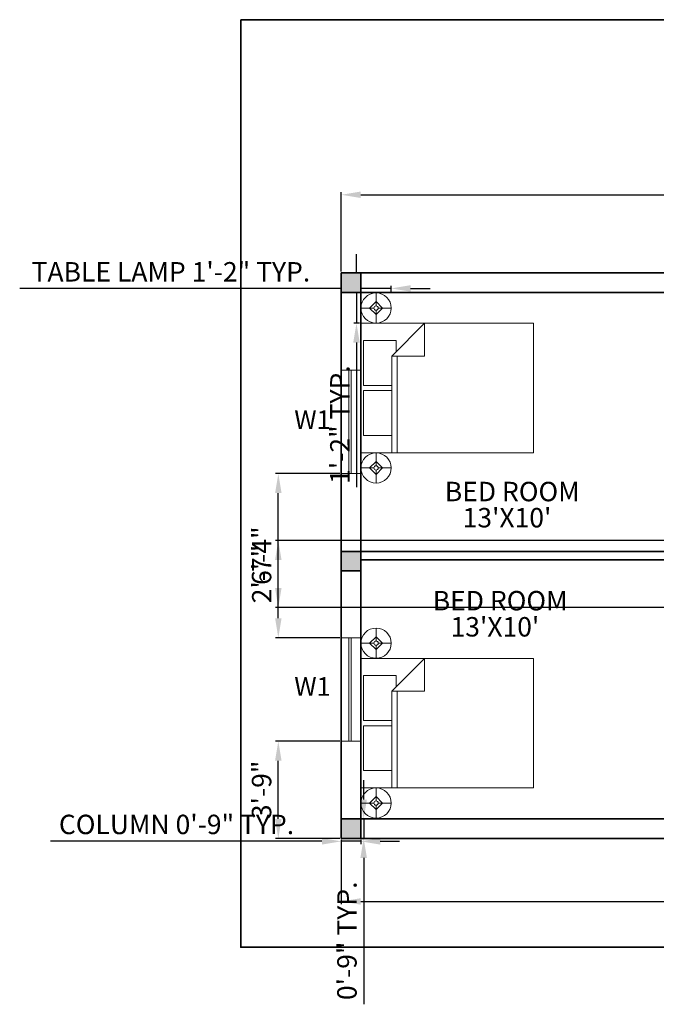
# Model space of a CAD drawing. Units: inches. Extents: x -281 to 2337, y 1647 to 2113.
# Tile 1 of 6: x 935 to 1230, y 1647 to 2103. Entities that reach past the tile are written whole.
import ezdxf

# ---------------------------------------------------------------- set-up
doc = ezdxf.new("R2010")
doc.units = ezdxf.units.IN
for name, color, linetype, lineweight in [('A-ANNO-DIMS', 242, 'Continuous', 18), ('A-ANNO-IDEN', 11, 'Continuous', 18), ('A-ANNO-TTLB', 7, 'Continuous', 35), ('A-AREA-IDEN', 7, 'Continuous', 18), ('A-COLS', 1, 'Continuous', 35), ('A-FURN', 8, 'Continuous', 18), ('A-GLAZ', 3, 'Continuous', 18), ('A-WALL', 7, 'Continuous', 35)]:
    doc.layers.add(name, color=color, linetype=linetype, lineweight=lineweight)
doc.styles.get("Standard").update_dxf_attribs({"font": 'arial.ttf'})
doc.dimstyles.new('ISO-25', dxfattribs={"dimtxt": 9, "dimasz": 9, "dimexe": 1.25, "dimexo": 0.625, "dimgap": 2, "dimtad": 1, "dimdec": 1, "dimlunit": 4, "dimtxsty": 'Standard', "dimcen": 2.5, "dimadec": 0, "dimazin": 0, "dimtfac": 1, "dimtdec": 1, "dimtmove": 0, "dimatfit": 3, "dimfxl": 1, "dimarcsym": 0})

# ---------------------------------------------------------------- blocks, each defined once
blk = doc.blocks.new('Bed - Queen')
for p, q in [((0, -80.00003), (0, 0)), ((0, 0), (59.99999, 0)), ((59.99999, 0), (59.99999, -80.00003)), ((7.99999, -1.2), (28.79998, -1.2)), ((7.99999, -14.4), (7.99999, -1.2)), ((28.79998, -1.2), (28.79998, -14.4)), ((31.19999, -1.2), (51.99999, -1.2)), ((31.19999, -14.4), (31.19999, -1.2)), ((51.99999, -1.2), (51.99999, -16.4)), ((0, -14.4), (44.8, -14.4)), ((44.8, -16.8), (0, -16.8)), ((59.99999, -29.6), (44.8, -14.4)), ((44.8, -14.4), (44.8, -29.6)), ((51.99999, -16.4), (46.79936, -16.4)), ((44.8, -29.6), (59.99999, -29.6)), ((59.99999, -80.00003), (0, -80.00003))]:
    blk.add_line(p, q)
blk = doc.blocks.new('Lamp - Table')
for p, q in [((0, 7), (0, 1)), ((-1, 0), (-7, 0)), ((0, 3), (-3, 0)), ((-3, 0), (0, -3)), ((3, 0), (0, 3)), ((0, -3), (3, 0)), ((1, 0), (7, 0)), ((0, -1), (0, -7))]:
    blk.add_line(p, q)
for radius in [7, 1]:
    blk.add_circle((0, 0), radius)
blk = doc.blocks.new('*D8')
at = {"layer": 'A-ANNO-DIMS', "color": 0, "lineweight": -2, "transparency": 16777216}
for p, q in [((1084.42, 1986.77), (1084.42, 2023.6)), ((1093.42, 2022.35), (1569.42, 2022.35)), ((1578.42, 1986.77), (1578.42, 2023.6))]:
    blk.add_line(p, q, dxfattribs=at)
at = {"layer": 'A-ANNO-DIMS', "color": 0, "transparency": 16777216}
for points in [[(1093.42, 2023.85), (1093.42, 2020.85), (1084.42, 2022.35)], [(1569.42, 2023.85), (1569.42, 2020.85), (1578.42, 2022.35)]]:
    blk.add_solid(points, dxfattribs=at)
at = {"layer": 'Defpoints', "color": 0, "transparency": 16777216}
for p in [(1578.42, 2022.35), (1084.42, 1986.15), (1578.42, 1986.15)]:
    blk.add_point(p, dxfattribs=at)
at = {"layer": 'A-ANNO-DIMS', "color": 0, "transparency": 16777216, "insert": (1331.42, 2028.86), "char_height": 9, "attachment_point": 5}
blk.add_mtext('41\'-2"', dxfattribs=at)
blk = doc.blocks.new('COL-9x9')
h = blk.add_hatch(color=256)
h.dxf.hatch_style = 1
h.paths.add_polyline_path([(9, 9), (0, 9), (0, 0), (9, 0)])
for p, q in [((0, 9), (9, 9)), ((0, 0), (0, 9)), ((9, 9), (9, 0)), ((9, 0), (0, 0))]:
    blk.add_line(p, q)
blk = doc.blocks.new('WIN-W1-48')
for p, q in [((0, 48), (9, 48)), ((3.5, 0), (3.5, 48)), ((4.5, 0), (4.5, 48)), ((0, 0), (9, 0))]:
    blk.add_line(p, q)
blk = doc.blocks.new('*D17')
at = {"layer": 'A-ANNO-DIMS', "color": 0, "lineweight": -2, "transparency": 16777216}
for p, q in [((1075.42, 1722.8), (949.69, 1722.8)), ((1084.42, 1723.52), (1084.42, 1721.55)), ((1093.42, 1722.8), (1084.42, 1722.8)), ((1093.42, 1723.52), (1093.42, 1721.55)), ((1102.42, 1722.8), (1111.42, 1722.8))]:
    blk.add_line(p, q, dxfattribs=at)
at = {"layer": 'A-ANNO-DIMS', "color": 0, "transparency": 16777216}
for points in [[(1075.42, 1724.3), (1075.42, 1721.3), (1084.42, 1722.8)], [(1102.42, 1724.3), (1102.42, 1721.3), (1093.42, 1722.8)]]:
    blk.add_solid(points, dxfattribs=at)
at = {"layer": 'Defpoints', "color": 0, "transparency": 16777216}
for p in [(1084.42, 1724.15), (1084.42, 1722.8), (1093.42, 1724.15)]:
    blk.add_point(p, dxfattribs=at)
at = {"layer": 'A-ANNO-DIMS', "color": 0, "transparency": 16777216, "insert": (1008.06, 1729.46), "char_height": 9, "attachment_point": 5}
blk.add_mtext('COLUMN 0\'-9" TYP.', dxfattribs=at)
blk = doc.blocks.new('*D18')
at = {"layer": 'A-ANNO-DIMS', "color": 0, "lineweight": -2, "transparency": 16777216}
for p, q in [((1094.77, 1742.15), (1094.77, 1751.15)), ((1094.05, 1733.15), (1096.02, 1733.15)), ((1094.77, 1733.15), (1094.77, 1724.15)), ((1094.05, 1724.15), (1096.02, 1724.15)), ((1094.77, 1715.15), (1094.77, 1647.29))]:
    blk.add_line(p, q, dxfattribs=at)
at = {"layer": 'A-ANNO-DIMS', "color": 0, "transparency": 16777216}
for points in [[(1093.27, 1742.15), (1096.27, 1742.15), (1094.77, 1733.15)], [(1093.27, 1715.15), (1096.27, 1715.15), (1094.77, 1724.15)]]:
    blk.add_solid(points, dxfattribs=at)
at = {"layer": 'Defpoints', "color": 0, "transparency": 16777216}
for p in [(1093.42, 1733.15), (1093.42, 1724.15), (1094.77, 1724.15)]:
    blk.add_point(p, dxfattribs=at)
at = {"layer": 'A-ANNO-DIMS', "color": 0, "transparency": 16777216, "insert": (1088.18, 1676.72), "char_height": 9, "attachment_point": 5, "rotation": 90}
blk.add_mtext('0\'-9" TYP.', dxfattribs=at)
blk = doc.blocks.new('*D27')
at = {"layer": 'A-ANNO-DIMS', "color": 0, "lineweight": -2, "transparency": 16777216}
for p, q in [((1093.53, 1977.5), (1093.53, 1980.23)), ((1107.53, 1977.5), (1107.53, 1980.23)), ((1084.53, 1978.98), (935.39, 1978.98)), ((1107.53, 1978.98), (1093.53, 1978.98)), ((1116.53, 1978.98), (1125.53, 1978.98))]:
    blk.add_line(p, q, dxfattribs=at)
at = {"layer": 'A-ANNO-DIMS', "color": 0, "transparency": 16777216}
for points in [[(1084.53, 1980.48), (1084.53, 1977.48), (1093.53, 1978.98)], [(1116.53, 1980.48), (1116.53, 1977.48), (1107.53, 1978.98)]]:
    blk.add_solid(points, dxfattribs=at)
at = {"layer": 'Defpoints', "color": 0, "transparency": 16777216}
for p in [(1093.53, 1978.98), (1093.53, 1976.88), (1107.53, 1976.88)]:
    blk.add_point(p, dxfattribs=at)
at = {"layer": 'A-ANNO-DIMS', "color": 0, "transparency": 16777216, "insert": (1005.46, 1985.5), "char_height": 9, "attachment_point": 5}
blk.add_mtext('TABLE LAMP 1\'-2" TYP.', dxfattribs=at)
blk = doc.blocks.new('*D28')
at = {"layer": 'A-ANNO-DIMS', "color": 0, "lineweight": -2, "transparency": 16777216}
for p, q in [((1091.43, 1985.88), (1091.43, 1994.88)), ((1092.91, 1976.88), (1090.18, 1976.88)), ((1091.43, 1976.88), (1091.43, 1962.88)), ((1092.91, 1962.88), (1090.18, 1962.88)), ((1091.43, 1953.88), (1091.43, 1886.87))]:
    blk.add_line(p, q, dxfattribs=at)
at = {"layer": 'A-ANNO-DIMS', "color": 0, "transparency": 16777216}
for points in [[(1089.93, 1985.88), (1092.93, 1985.88), (1091.43, 1976.88)], [(1089.93, 1953.88), (1092.93, 1953.88), (1091.43, 1962.88)]]:
    blk.add_solid(points, dxfattribs=at)
at = {"layer": 'Defpoints', "color": 0, "transparency": 16777216}
for p in [(1093.53, 1976.88), (1091.43, 1962.88), (1093.53, 1962.88)]:
    blk.add_point(p, dxfattribs=at)
at = {"layer": 'A-ANNO-DIMS', "color": 0, "transparency": 16777216, "insert": (1084.91, 1915.87), "char_height": 9, "attachment_point": 5, "rotation": 90}
blk.add_mtext('1\'-2" TYP.', dxfattribs=at)
blk = doc.blocks.new('*D42')
at = {"layer": 'A-ANNO-DIMS', "color": 0, "lineweight": -2, "transparency": 16777216}
for p, q in [((1084.42, 1723.52), (1084.42, 1693.7)), ((1605.42, 1723.52), (1605.42, 1693.7)), ((1093.42, 1694.95), (1596.42, 1694.95))]:
    blk.add_line(p, q, dxfattribs=at)
at = {"layer": 'A-ANNO-DIMS', "color": 0, "transparency": 16777216}
for points in [[(1093.42, 1696.45), (1093.42, 1693.45), (1084.42, 1694.95)], [(1596.42, 1696.45), (1596.42, 1693.45), (1605.42, 1694.95)]]:
    blk.add_solid(points, dxfattribs=at)
at = {"layer": 'Defpoints', "color": 0, "transparency": 16777216}
for p in [(1084.42, 1724.15), (1605.42, 1724.15), (1605.42, 1694.95)]:
    blk.add_point(p, dxfattribs=at)
at = {"layer": 'A-ANNO-DIMS', "color": 0, "transparency": 16777216, "insert": (1344.92, 1701.55), "char_height": 9, "attachment_point": 5}
blk.add_mtext('43\'-5"', dxfattribs=at)
blk = doc.blocks.new('*D49')
at = {"layer": 'A-ANNO-DIMS', "color": 0, "lineweight": -2, "transparency": 16777216}
for p, q in [((1083.8, 1769.15), (1053.97, 1769.15)), ((1055.22, 1733.15), (1055.22, 1760.15)), ((1083.8, 1724.15), (1053.97, 1724.15))]:
    blk.add_line(p, q, dxfattribs=at)
at = {"layer": 'A-ANNO-DIMS', "color": 0, "transparency": 16777216}
for points in [[(1053.72, 1760.15), (1056.72, 1760.15), (1055.22, 1769.15)], [(1053.72, 1733.15), (1056.72, 1733.15), (1055.22, 1724.15)]]:
    blk.add_solid(points, dxfattribs=at)
at = {"layer": 'Defpoints', "color": 0, "transparency": 16777216}
for p in [(1055.22, 1769.15), (1084.42, 1769.15), (1084.42, 1724.15)]:
    blk.add_point(p, dxfattribs=at)
at = {"layer": 'A-ANNO-DIMS', "color": 0, "transparency": 16777216, "insert": (1048.63, 1746.65), "char_height": 9, "attachment_point": 5, "rotation": 90}
blk.add_mtext('3\'-9"', dxfattribs=at)
blk = doc.blocks.new('*D50')
at = {"layer": 'A-ANNO-DIMS', "color": 0, "lineweight": -2, "transparency": 16777216}
for p, q in [((1083.8, 1893.15), (1053.97, 1893.15)), ((1055.22, 1826.15), (1055.22, 1884.15)), ((1083.8, 1817.15), (1053.97, 1817.15))]:
    blk.add_line(p, q, dxfattribs=at)
at = {"layer": 'A-ANNO-DIMS', "color": 0, "transparency": 16777216}
for points in [[(1053.72, 1884.15), (1056.72, 1884.15), (1055.22, 1893.15)], [(1053.72, 1826.15), (1056.72, 1826.15), (1055.22, 1817.15)]]:
    blk.add_solid(points, dxfattribs=at)
at = {"layer": 'Defpoints', "color": 0, "transparency": 16777216}
for p in [(1055.22, 1893.15), (1084.42, 1893.15), (1084.42, 1817.15)]:
    blk.add_point(p, dxfattribs=at)
at = {"layer": 'A-ANNO-DIMS', "color": 0, "transparency": 16777216, "insert": (1048.63, 1855.15), "char_height": 9, "attachment_point": 5, "rotation": 90}
blk.add_mtext('6\'-4"', dxfattribs=at)
blk = doc.blocks.new('*D57')
at = {"layer": 'A-ANNO-DIMS', "color": 0, "lineweight": -2, "transparency": 16777216}
for p, q in [((1577.8, 1862.15), (1053.97, 1862.15)), ((1055.22, 1840.15), (1055.22, 1853.15)), ((1577.8, 1831.15), (1053.97, 1831.15))]:
    blk.add_line(p, q, dxfattribs=at)
at = {"layer": 'A-ANNO-DIMS', "color": 0, "transparency": 16777216}
for points in [[(1053.72, 1853.15), (1056.72, 1853.15), (1055.22, 1862.15)], [(1053.72, 1840.15), (1056.72, 1840.15), (1055.22, 1831.15)]]:
    blk.add_solid(points, dxfattribs=at)
at = {"layer": 'Defpoints', "color": 0, "transparency": 16777216}
for p in [(1055.22, 1862.15), (1578.42, 1862.15), (1578.42, 1831.15)]:
    blk.add_point(p, dxfattribs=at)
at = {"layer": 'A-ANNO-DIMS', "color": 0, "transparency": 16777216, "insert": (1048.71, 1846.65), "char_height": 9, "attachment_point": 5, "rotation": 90}
blk.add_mtext('2\'-7"', dxfattribs=at)

msp = doc.modelspace()

# ---------------------------------------------------------------- linework, layer by layer
at = {"layer": 'A-ANNO-TTLB'}
msp.add_lwpolyline([(1037.79, 2103.48), (2323.1, 2103.48), (2323.1, 1673.73), (1037.79, 1673.73)], close=True, dxfattribs=at)
at = {"layer": 'A-WALL'}
for p, q in [((1084.42, 1986.15), (1605.42, 1986.15)), ((1084.42, 1724.15), (1084.42, 1986.15)), ((1093.42, 1977.15), (1601.42, 1977.15)), ((1093.42, 1733.15), (1093.42, 1977.15)), ((1253.42, 1857.15), (1084.42, 1857.15)), ((1253.42, 1853.15), (1093.42, 1853.15)), ((1249.42, 1733.15), (1093.42, 1733.15)), ((1605.42, 1724.15), (1084.42, 1724.15))]:
    msp.add_line(p, q, dxfattribs=at)

# ---------------------------------------------------------------- block references
at = {"layer": 'A-COLS', "rotation": 180}
for p in [(1093.42, 1986.15), (1093.42, 1857.15), (1093.42, 1733.15)]:
    msp.add_blockref('COL-9x9', p, dxfattribs=at)
at = {"layer": 'A-FURN'}
for name, p, rotation in [('Lamp - Table', (1100.53, 1969.88), 180), ('Bed - Queen', (1093.42, 1902.85), 89.99999999999999), ('Lamp - Table', (1100.53, 1895.8), 180), ('Lamp - Table', (1100.53, 1814.61), 180), ('Bed - Queen', (1093.42, 1747.58), 89.99999999999999), ('Lamp - Table', (1100.53, 1740.53), 180)]:
    msp.add_blockref(name, p, dxfattribs=dict(at, rotation=rotation))
at = {"layer": 'A-GLAZ'}
for p in [(1084.42, 1893.15), (1084.42, 1769.15)]:
    msp.add_blockref('WIN-W1-48', p, dxfattribs=at)

# ---------------------------------------------------------------- texts
at = {"layer": 'A-ANNO-IDEN'}
for p in [(1062.63, 1913.82), (1062.63, 1790.24)]:
    msp.add_text('W1', height=8.623, dxfattribs=at).set_placement(p)
at = {"layer": 'A-AREA-IDEN'}
for s, p in [('BED ROOM', (1132.37, 1880.36)), ("   13'X10'", (1132.37, 1868.25)), ('BED ROOM', (1126.77, 1829.8)), ("   13'X10'", (1126.77, 1817.69))]:
    msp.add_text(s, height=9, dxfattribs=at).set_placement(p)

# ---------------------------------------------------------------- dimensions: what is measured, and where the dimension line sits
at = {"layer": 'A-ANNO-DIMS'}
for base, p1, p2, override, picture, middle in [((1578.42, 2022.35), (1084.42, 1986.15), (1578.42, 1986.15), {"dimclrd": 0, "dimclre": 0, "dimclrt": 0}, '*D8', (1331.42, 2028.86)), ((1605.42, 1694.95), (1084.42, 1724.15), (1605.42, 1724.15), {"dimdec": 1, "dimlfac": 1, "dimrnd": 0, "dimzin": 1, "dimdsep": 46, "dimlunit": 4, "dimfrac": 2}, '*D42', (1344.92, 1701.55))]:
    dim = msp.add_linear_dim(base=base, p1=p1, p2=p2, dimstyle='ISO-25', override=override, dxfattribs=at)
    dim.commit()
    dim.dimension.update_dxf_attribs({"geometry": picture, "text_midpoint": middle})
for base, p1, p2, angle, text, picture, middle in [((1093.53, 1978.98), (1107.53, 1976.88), (1093.53, 1976.88), 180, 'TABLE LAMP <> TYP.', '*D27', (1005.46, 1985.5)), ((1091.43, 1962.88), (1093.53, 1976.88), (1093.53, 1962.88), 270, '<> TYP.', '*D28', (1084.91, 1915.87)), ((1084.42, 1722.8), (1093.42, 1724.15), (1084.42, 1724.15), 180, 'COLUMN <> TYP.', '*D17', (1008.06, 1729.46)), ((1094.77, 1724.15), (1093.42, 1733.15), (1093.42, 1724.15), 270, '<> TYP.', '*D18', (1088.18, 1676.72))]:
    dim = msp.add_linear_dim(base=base, p1=p1, p2=p2, angle=angle, text=text, dimstyle='ISO-25', override={"dimdec": 1, "dimlfac": 1, "dimrnd": 0, "dimzin": 1, "dimdsep": 46, "dimlunit": 4, "dimfrac": 2}, dxfattribs=at)
    dim.commit()
    dim.dimension.update_dxf_attribs({"geometry": picture, "text_midpoint": middle})
for base, p1, p2, picture, middle in [((1055.22, 1893.15), (1084.42, 1817.15), (1084.42, 1893.15), '*D50', (1048.63, 1855.15)), ((1055.22, 1862.15), (1578.42, 1831.15), (1578.42, 1862.15), '*D57', (1048.71, 1846.65)), ((1055.22, 1769.15), (1084.42, 1724.15), (1084.42, 1769.15), '*D49', (1048.63, 1746.65))]:
    dim = msp.add_linear_dim(base=base, p1=p1, p2=p2, angle=90, dimstyle='ISO-25', override={"dimdec": 1, "dimlfac": 1, "dimrnd": 0, "dimzin": 1, "dimdsep": 46, "dimlunit": 4, "dimfrac": 2}, dxfattribs=at)
    dim.commit()
    dim.dimension.update_dxf_attribs({"geometry": picture, "text_midpoint": middle})

doc.saveas('drawing.dxf')
